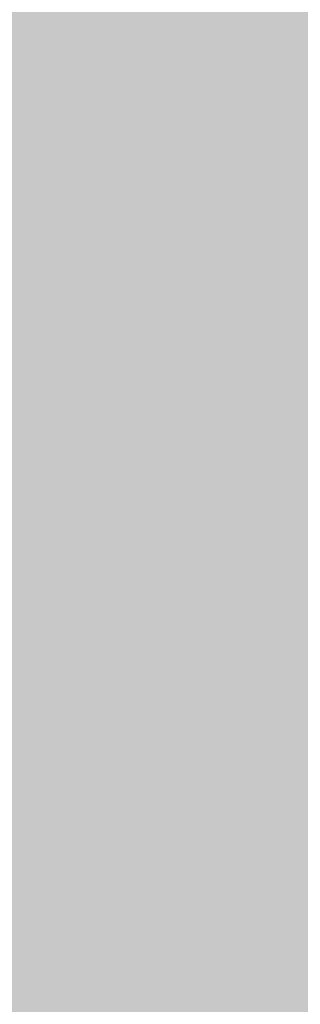
# Model space of a CAD drawing. Units: inches. Extents: x 2083 to 3317, y 1141 to 2115.
# Tile 187 of 256: x 3126.8176 to 3126.8914, y 1263.3548 to 1263.6134. Entities that reach past the tile are written whole.
import ezdxf

# ---------------------------------------------------------------- set-up
doc = ezdxf.new("R2010")
doc.units = ezdxf.units.IN
doc.layers.add('A-ANNO-DIMS', color=2, linetype='Continuous', lineweight=18)
doc.layers.add('A-WALL-PATT', color=251, linetype='Continuous', lineweight=13, true_color=0x636466)
doc.styles.get("Standard").update_dxf_attribs({"font": 'arial.ttf'})
doc.dimstyles.new('ISO-25', dxfattribs={"dimtxt": 12, "dimasz": 12, "dimexe": 1.25, "dimexo": 0.625, "dimtad": 1, "dimlunit": 3, "dimtxsty": 'Standard', "dimcen": 2.5, "dimadec": 0, "dimazin": 0, "dimtfac": 1, "dimtmove": 0, "dimatfit": 3, "dimfxl": 1, "dimarcsym": 0})

# ---------------------------------------------------------------- blocks, each defined once
blk = doc.blocks.new('*D26')
at = {"layer": 'A-ANNO-DIMS', "color": 0, "lineweight": -2, "transparency": 16777216}
for p, q in [((3088.98584, 1274.91509), (3088.98584, 1270.95196)), ((3111.24004, 1274.91509), (3111.24004, 1270.95196)), ((3076.98584, 1272.20196), (2840.26245, 1272.20196)), ((3111.24004, 1272.20196), (3088.98584, 1272.20196)), ((3123.24004, 1272.20196), (3135.24004, 1272.20196))]:
    blk.add_line(p, q, dxfattribs=at)
at = {"layer": 'A-ANNO-DIMS', "color": 0, "transparency": 16777216}
for points in [[(3076.98584, 1274.20196), (3076.98584, 1270.20196), (3088.98584, 1272.20196)], [(3123.24004, 1274.20196), (3123.24004, 1270.20196), (3111.24004, 1272.20196)]]:
    blk.add_solid(points, dxfattribs=at)
at = {"layer": 'Defpoints', "color": 0, "transparency": 16777216}
for p in [(3088.98584, 1275.54009), (3111.24004, 1275.54009), (3088.98584, 1272.20196)]:
    blk.add_point(p, dxfattribs=at)
at = {"layer": 'A-ANNO-DIMS', "color": 0, "transparency": 16777216, "insert": (2952.62415, 1279.0316), "char_height": 12, "attachment_point": 5}
blk.add_mtext('NIGHTSTAND 1\'-10 1/2" TYP.', dxfattribs=at)
blk = doc.blocks.new('*D27')
at = {"layer": 'A-ANNO-DIMS', "color": 0, "lineweight": -2, "transparency": 16777216}
for p, q in [((3114.57817, 1309.79428), (3114.57817, 1321.79428)), ((3111.86504, 1297.79428), (3115.82817, 1297.79428)), ((3114.57817, 1297.79428), (3114.57817, 1275.54009)), ((3111.86504, 1275.54009), (3115.82817, 1275.54009)), ((3114.57817, 1263.54009), (3114.57817, 1140.98859))]:
    blk.add_line(p, q, dxfattribs=at)
at = {"layer": 'A-ANNO-DIMS', "color": 0, "transparency": 16777216}
for points in [[(3112.57817, 1309.79428), (3116.57817, 1309.79428), (3114.57817, 1297.79428)], [(3112.57817, 1263.54009), (3116.57817, 1263.54009), (3114.57817, 1275.54009)]]:
    blk.add_solid(points, dxfattribs=at)
at = {"layer": 'Defpoints', "color": 0, "transparency": 16777216}
for p in [(3111.24004, 1297.79428), (3111.24004, 1275.54009), (3114.57817, 1275.54009)]:
    blk.add_point(p, dxfattribs=at)
at = {"layer": 'A-ANNO-DIMS', "color": 0, "transparency": 16777216, "insert": (3107.74853, 1196.26434), "char_height": 12, "attachment_point": 5, "rotation": 90}
blk.add_mtext('1\'-10 1/2" TYP.', dxfattribs=at)

msp = doc.modelspace()

# ---------------------------------------------------------------- hatches: boundary and pattern name
at = {"layer": 'A-WALL-PATT'}
h = msp.add_hatch(color=256, dxfattribs=at)
h.dxf.hatch_style = 1
h.paths.add_polyline_path([(3126.95978, 2020.76136), (2748.95978, 2020.76136), (2604.95978, 2020.76136), (2226.95978, 2020.76136), (2226.95978, 1702.76136), (2466.95978, 1702.76136), (2466.95978, 1582.76136), (2418.95978, 1582.76136), (2418.95978, 1477.76136), (2226.95978, 1477.76136), (2226.95978, 1263.26136), (2544.95978, 1263.26136), (2544.95978, 1411.76136), (2604.95978, 1411.76136), (2685.95978, 1411.76136), (2685.95978, 1420.76136), (2604.95978, 1420.76136), (2604.95978, 1573.76136), (2604.95978, 1702.76136), (2604.95978, 2011.76136), (2748.95978, 2011.76136), (2748.95978, 1702.76136), (2862.95978, 1702.76136), (2862.95978, 1621.76136), (2871.95978, 1621.76136), (2871.95978, 1702.76136), (2883.95978, 1702.76136), (2883.95978, 1706.93946, -0.026459), (2883.95978, 1711.76136), (2757.95978, 1711.76136), (2757.95978, 1807.76136), (2787.95978, 1807.76136), (2787.95978, 1812.26136), (2757.95978, 1812.26136), (2757.95978, 2011.76136), (2877.95978, 2011.76136), (2877.95978, 1812.26136), (2847.95978, 1812.26136), (2847.95978, 1807.76136), (2889.83574, 1807.76136), (2889.83574, 1812.26136), (2882.45978, 1812.26136), (2882.45978, 2011.76136), (3117.95978, 2011.76136), (3117.95978, 1812.26136), (2937.83574, 1812.26136), (2937.83574, 1807.76136), (2995.70978, 1807.76136), (2995.70978, 1796.11767), (3000.20978, 1796.11767), (3000.20978, 1807.76136), (3117.95978, 1807.76136), (3117.95978, 1711.76136), (3000.20978, 1711.76136), (3000.20978, 1760.11767), (2998.5727, 1760.11767, -0.020711), (2995.70978, 1760.11767), (2995.70978, 1711.76136), (2931.95978, 1711.76136), (2931.95978, 1702.76136), (3126.95978, 1702.76136)])
h.paths.add_polyline_path([(2471.45978, 2011.76136), (2471.45978, 1810.01136), (2462.71694, 1810.01136), (2462.71694, 1805.51136), (2505.95978, 1805.51136), (2505.95978, 1810.01136), (2475.95978, 1810.01136), (2475.95978, 2011.76136), (2595.95978, 2011.76136), (2595.95978, 1810.01136), (2565.95978, 1810.01136), (2565.95978, 1805.51136), (2595.95978, 1805.51136), (2595.95978, 1711.76136), (2235.95978, 1711.76136), (2235.95978, 1805.51136), (2353.70978, 1805.51136), (2353.70978, 1796.05416), (2358.20978, 1796.05416), (2358.20978, 1805.51136), (2414.71694, 1805.51136), (2414.71694, 1810.01136), (2235.95978, 1810.01136), (2235.95978, 2011.76136)], flags=16)
h.paths.add_polyline_path([(2270.20473, 1994.61001), (2270.20473, 1970.61001), (2246.20473, 1970.61001), (2246.20473, 1994.61001)], flags=0)
edge = h.paths.add_edge_path(flags=0)
edge.add_ellipse((2332.02739, 1899.79818), major_axis=(-3.04299, 3.04299), ratio=0.1682525, start_angle=-161.33217, end_angle=-156.30711, ccw=False)
edge.add_ellipse((2333.08204, 1898.74353), major_axis=(-1.05465, 1.05465), ratio=0.4535321, start_angle=-123.37102, end_angle=-94.15911)
edge = h.paths.add_edge_path(flags=0)
edge.add_ellipse((2332.02739, 1968.87629), major_axis=(3.04299, 3.04299), ratio=0.1682525, start_angle=18.66783, end_angle=23.69289)
edge.add_spline(control_points=[(2332.9256, 1970.6911), (2332.22677, 1970.3361), (2330.89371, 1969.65891), (2328.41308, 1970.93214), (2327.20393, 1967.74871), (2324.7096, 1969.95559), (2322.53282, 1967.01235), (2320.01285, 1971.29581), (2317.68031, 1968.15784), (2316.04053, 1967.10205), (2315.4269, 1966.8096)], knot_values=[0, 0, 0, 0, 2.267059, 4.324559, 6.685584, 8.878641, 11.121502, 14.300359, 17.755284, 19.732645, 19.732645, 19.732645, 19.732645], degree=3, periodic=0)
edge.add_ellipse((2332.02739, 1968.87629), major_axis=(3.04299, 3.04299), ratio=0.1682525, start_angle=18.66783, end_angle=23.69289, ccw=False)
edge.add_ellipse((2333.08204, 1969.93094), major_axis=(1.05465, 1.05465), ratio=0.4535321, start_angle=56.62898, end_angle=85.84089, ccw=False)
edge = h.paths.add_edge_path(flags=0)
edge.add_spline(control_points=[(2296.42829, 1967.98791), (2293.6278, 1965.33631), (2287.70362, 1959.72709), (2299.74386, 1949.9957), (2294.53259, 1935.66853), (2290.57323, 1920.60351), (2293.39412, 1909.97369), (2296.18541, 1904.96654)], knot_values=[0.099185, 0.099185, 0.099185, 0.099185, 0.345301, 0.619822, 0.982653, 1.386093, 1.810555, 1.810555, 1.810555, 1.810555], degree=3, periodic=0)
edge.add_spline(control_points=[(2296.18541, 1904.96654), (2297.38358, 1902.6193), (2298.00097, 1901.94931), (2298.55297, 1901.46815)], knot_values=[0.006246, 0.006246, 0.006246, 0.006246, 0.055476, 0.055476, 0.055476, 0.055476], degree=3, periodic=0)
edge.add_spline(control_points=[(2298.55297, 1901.46815), (2297.25861, 1900.92322), (2295.22529, 1900.23213), (2293.06023, 1900.61421), (2292.10142, 1900.78841), (2292.08958, 1900.79057)], knot_values=[0.312835, 0.312835, 0.312835, 0.312835, 0.40178, 0.474987, 0.475903, 0.475903, 0.475903, 0.475903], degree=3, periodic=0)
edge.add_arc((2292.79365, 1904.66411), 3.93701, 215.4209, 259.69818, ccw=False)
edge.add_spline(control_points=[(2289.58531, 1902.3823), (2289.47665, 1902.53509), (2289.36848, 1902.68804), (2289.26086, 1902.84117)], knot_values=[0.102872, 0.102872, 0.102872, 0.102872, 0.116896, 0.116896, 0.116896, 0.116896], degree=3, periodic=0)
edge.add_spline(control_points=[(2289.26086, 1902.84117), (2288.6866, 1902.55019), (2287.64005, 1902.0199), (2285.88134, 1901.87395), (2283.85297, 1901.50435), (2281.71999, 1899.71054), (2278.46699, 1899.49294), (2276.15714, 1901.8832), (2272.25895, 1899.80407), (2267.77761, 1901.84318), (2262.24388, 1900.18403), (2257.41493, 1901.78206), (2254.31837, 1900.72612), (2253.17828, 1900.33734)], knot_values=[0, 0, 0, 0, 1.907977, 3.477176, 5.261074, 7.972851, 11.680248, 13.717921, 16.939592, 22.789562, 27.502503, 33.595215, 37.145618, 37.145618, 37.145618, 37.145618], degree=3, periodic=0)
edge.add_line((2253.17828, 1900.33734), (2250.24424, 1902.84117))
edge.add_line((2250.24424, 1902.84117), (2250.24424, 1965.8333))
edge.add_line((2250.24424, 1965.8333), (2253.17828, 1968.33712))
edge.add_spline(control_points=[(2253.17828, 1968.33712), (2254.31837, 1967.94835), (2257.41493, 1966.89241), (2262.24388, 1968.49043), (2267.77761, 1966.83128), (2271.52673, 1968.53722), (2273.87591, 1967.82829), (2274.2067, 1967.72764)], knot_values=[0, 0, 0, 0, 0.09018, 0.244935, 0.364644, 0.513233, 0.537855, 0.537855, 0.537855, 0.537855], degree=3, periodic=0)
edge.add_arc((2274.35289, 1963.79335), 3.93701, 72.05113, 92.12795, ccw=False)
edge.add_arc((2281.29693, 1985.23), 18.5963, 252.051134, 288.565722)
edge.add_arc((2292.31672, 1956.02888), 12.64608, 71.026788, 113.778218, ccw=False)
edge = h.paths.add_edge_path(flags=0)
edge.add_spline(control_points=[(2274.89941, 1951.85619), (2275.06616, 1951.61659), (2275.23269, 1951.37659), (2275.39799, 1951.13585)], knot_values=[1.409916, 1.409916, 1.409916, 1.409916, 1.43159, 1.43159, 1.43159, 1.43159], degree=3, periodic=0)
edge.add_spline(control_points=[(2275.39799, 1951.13585), (2275.79211, 1950.56189), (2276.17923, 1949.98377), (2276.54555, 1949.3971)], knot_values=[1.358238, 1.358238, 1.358238, 1.358238, 1.409916, 1.409916, 1.409916, 1.409916], degree=3, periodic=0)
edge.add_line((2276.54555, 1949.3971), (2277.43729, 1947.86218))
edge.add_spline(control_points=[(2277.43729, 1947.86218), (2276.30383, 1945.67311), (2274.6397, 1942.42688), (2274.63161, 1938.0939), (2272.79912, 1930.85155), (2274.35643, 1943.89705), (2275.94768, 1947.92336), (2276.54555, 1949.3971)], knot_values=[0.005632, 0.005632, 0.005632, 0.005632, 0.186014, 0.266002, 0.357087, 0.59639, 0.739732, 0.739732, 0.739732, 0.739732], degree=3, periodic=0)
edge.add_spline(control_points=[(2276.54555, 1949.3971), (2276.17923, 1949.98377), (2275.79211, 1950.56189), (2275.39799, 1951.13585)], knot_values=[1.358238, 1.358238, 1.358238, 1.358238, 1.409916, 1.409916, 1.409916, 1.409916], degree=3, periodic=0)
edge.add_spline(control_points=[(2275.39799, 1951.13585), (2274.9425, 1950.08045), (2274.20776, 1948.02527), (2273.9346, 1944.85148), (2272.46853, 1937.62749), (2273.46622, 1945.69647), (2274.70062, 1951.05947), (2274.89941, 1951.85619)], knot_values=[0.104364, 0.104364, 0.104364, 0.104364, 0.189636, 0.269624, 0.36071, 0.600013, 0.644622, 0.644622, 0.644622, 0.644622], degree=3, periodic=0)
h.paths.add_polyline_path([(2269.16751, 1963.12757, -0.357527), (2268.17063, 1960.97637, -0.092561), (2268.17063, 1939.43632, -0.357527), (2269.16751, 1937.28512, -0.357527), (2267.01631, 1938.282, -0.164785), (2254.68558, 1938.282, -0.357527), (2252.53438, 1937.28512, -0.357527), (2253.53126, 1939.43632, -0.092561), (2253.53126, 1960.97637, -0.357527), (2252.53438, 1963.12757, -0.357527), (2254.68558, 1962.13069, -0.164785), (2267.01631, 1962.13069, -0.357527)], flags=0)
h.paths.add_polyline_path([(2248.87407, 1967.8018), (2248.87407, 1957.02771), (2249.45778, 1957.02771), (2249.45778, 1911.64676), (2248.87407, 1911.64676), (2248.87407, 1900.87267), (2246.51186, 1900.87267, 0.197327), (2244.14966, 1902.45687), (2244.14966, 1966.21759, 0.197327), (2246.51186, 1967.8018)], flags=0)
h.paths.add_polyline_path([(2269.16751, 1931.38934, -0.357527), (2268.17063, 1929.23814, -0.092561), (2268.17063, 1907.6981, -0.357527), (2269.16751, 1905.54689, -0.357527), (2267.01631, 1906.54377, -0.164785), (2254.68558, 1906.54377, -0.357527), (2252.53438, 1905.54689, -0.357527), (2253.53126, 1907.6981, -0.092561), (2253.53126, 1929.23814, -0.357527), (2252.53438, 1931.38934, -0.357527), (2254.68558, 1930.39246, -0.164785), (2267.01631, 1930.39246, -0.357527)], flags=0)
edge = h.paths.add_edge_path(flags=0)
edge.add_spline(control_points=[(2276.19686, 1906.7237), (2276.16814, 1909.02893), (2276.11405, 1913.37185), (2270.59842, 1924.92498), (2273.90517, 1919.01278), (2275.92171, 1916.26206), (2275.47457, 1912.40215), (2277.25787, 1910.38062), (2276.69604, 1908.22504), (2276.64622, 1906.81302), (2276.61782, 1906.00841)], knot_values=[0, 0, 0, 0, 8.61026, 16.221274, 18.843057, 23.804898, 27.440828, 29.356102, 31.203478, 33.650687, 33.650687, 33.650687, 33.650687], degree=3, periodic=0)
edge.add_spline(control_points=[(2276.61782, 1906.00841), (2276.62331, 1905.62414), (2276.49774, 1904.62866), (2275.44178, 1903.85473), (2274.93731, 1903.08045), (2274.85908, 1902.84117)], knot_values=[0.156488, 0.156488, 0.156488, 0.156488, 0.184398, 0.231376, 0.250598, 0.250598, 0.250598, 0.250598], degree=3, periodic=0)
edge.add_line((2274.85908, 1902.84117), (2276.50598, 1902.84117))
edge.add_spline(control_points=[(2276.50598, 1902.84117), (2276.78831, 1903.08494), (2277.66507, 1904.1252), (2278.24954, 1904.34074), (2277.65387, 1908.52739), (2278.15567, 1906.22781), (2278.10046, 1905.28595), (2278.84667, 1904.06901), (2277.85679, 1903.41495), (2277.87419, 1902.99105), (2277.90356, 1902.84117)], knot_values=[0.059574, 0.059574, 0.059574, 0.059574, 0.080753, 0.103741, 0.16972, 0.176036, 0.207137, 0.240474, 0.262341, 0.27366, 0.27366, 0.27366, 0.27366], degree=3, periodic=0)
edge.add_line((2277.90356, 1902.84117), (2280.02983, 1902.84117))
edge.add_spline(control_points=[(2280.02983, 1902.84117), (2279.88822, 1903.0884), (2279.49926, 1903.98155), (2280.15228, 1905.93935), (2278.10362, 1909.65776), (2279.76239, 1907.18529), (2280.3279, 1904.87486), (2280.48511, 1903.48959), (2281.46327, 1903.24943), (2281.75834, 1902.9365), (2281.83404, 1902.84117)], knot_values=[0.013856, 0.013856, 0.013856, 0.013856, 0.034874, 0.088867, 0.107879, 0.126738, 0.158714, 0.193757, 0.217487, 0.226722, 0.226722, 0.226722, 0.226722], degree=3, periodic=0)
edge.add_spline(control_points=[(2281.83404, 1902.84117), (2281.78753, 1902.8267), (2281.64702, 1902.78299), (2281.39553, 1902.85949), (2281.08808, 1902.98524), (2280.72068, 1903.0609), (2280.33345, 1903.02573), (2280.12477, 1902.89888), (2280.02983, 1902.84117)], knot_values=[0, 0, 0, 0, 0.14413, 0.435517, 0.749276, 1.153046, 1.548371, 1.878348, 1.878348, 1.878348, 1.878348], degree=3, periodic=0)
edge.add_line((2280.02983, 1902.84117), (2277.90356, 1902.84117))
edge.add_spline(control_points=[(2277.90356, 1902.84117), (2277.89286, 1902.79586), (2277.8654, 1902.67964), (2277.60748, 1902.68748), (2277.27405, 1902.8007), (2276.83792, 1902.61977), (2276.58381, 1902.78926), (2276.50598, 1902.84117)], knot_values=[0, 0, 0, 0, 0.127189, 0.326199, 0.628009, 1.24357, 1.515331, 1.515331, 1.515331, 1.515331], degree=3, periodic=0)
edge.add_line((2276.50598, 1902.84117), (2274.85908, 1902.84117))
edge.add_spline(control_points=[(2274.85908, 1902.84117), (2274.81444, 1902.89859), (2274.72513, 1903.01345), (2274.49348, 1903.11897), (2274.24429, 1902.96054), (2273.93712, 1903.18494), (2273.61404, 1902.98314), (2273.40832, 1902.88304), (2273.32225, 1902.84117)], knot_values=[0, 0, 0, 0, 0.21843, 0.436957, 0.687977, 0.990379, 1.398396, 1.69185, 1.69185, 1.69185, 1.69185], degree=3, periodic=0)
edge.add_spline(control_points=[(2273.32225, 1902.84117), (2273.61674, 1903.44569), (2274.274, 1904.53825), (2276.02724, 1904.5737), (2276.20696, 1906.58364), (2276.19686, 1906.7237)], knot_values=[0.012227, 0.012227, 0.012227, 0.012227, 0.059472, 0.106218, 0.134458, 0.134458, 0.134458, 0.134458], degree=3, periodic=0)
h.paths.add_polyline_path([(2270.77605, 1897.78983), (2270.77605, 1873.78983), (2246.77605, 1873.78983), (2246.77605, 1897.78983)], flags=0)
h.paths.add_polyline_path([(2353.70978, 1760.00506), (2353.70978, 1760.05416), (2358.20978, 1760.05416, -0.033729)], flags=0)
h.paths.add_polyline_path([(2321.81912, 1737.52919), (2341.99533, 1737.52919, -0.414214), (2343.20327, 1736.32124), (2343.20327, 1721.0206, -0.414214), (2341.99533, 1719.81265), (2321.81912, 1719.81265, -0.414214), (2320.61117, 1721.0206), (2320.61117, 1736.32124, -0.414214)], flags=0)
h.paths.add_polyline_path([(2324.23501, 1736.32124), (2339.57944, 1736.32124, -0.414214), (2341.99533, 1733.90535), (2341.99533, 1725.44973, -0.414214), (2339.57944, 1723.03384), (2333.68059, 1723.03384), (2333.84532, 1722.04547, -0.870646), (2335.4254, 1721.82589, -0.767327), (2333.92269, 1721.42324), (2331.29102, 1721.42324, -0.767327), (2329.78832, 1721.82589, -0.870646), (2331.3684, 1722.04547), (2331.53313, 1723.03384), (2324.23501, 1723.03384, -0.414214), (2321.81912, 1725.44973), (2321.81912, 1733.90535, -0.414214)], flags=0)
h.paths.add_polyline_path([(2570.48379, 1928.61544), (2589.68379, 1928.61544), (2590.16883, 1928.61544), (2590.16883, 1904.9934), (2570.48379, 1904.9934)], flags=0)
h.paths.add_polyline_path([(2574.44732, 1927.26382, -1), (2572.82884, 1927.26382, -1)], flags=0)
h.paths.add_polyline_path([(2573.08987, 1926.94088), (2573.92503, 1927.77604), (2574.14774, 1927.55333), (2573.31258, 1926.71817)], flags=0)
h.paths.add_polyline_path([(2578.77906, 1919.72962, -1), (2571.59166, 1919.72962, -1)], flags=0)
h.paths.add_polyline_path([(2578.38536, 1919.72962, -1), (2571.98536, 1919.72962, -1)], flags=0)
h.paths.add_polyline_path([(2331.59576, 1729.47622, -1), (2333.61795, 1729.47622, -1)], flags=0)
h.paths.add_polyline_path([(2578.03423, 1927.26382, -1), (2576.41574, 1927.26382, -1)], flags=0)
h.paths.add_polyline_path([(2576.68885, 1927.53109), (2576.91156, 1927.7538), (2577.74673, 1926.91863), (2577.52402, 1926.69592)], flags=0)
h.paths.add_polyline_path([(2578.13906, 1909.85954, -1), (2572.23166, 1909.85954, -1)], flags=0)
h.paths.add_polyline_path([(2577.74536, 1909.85954, -1), (2572.62536, 1909.85954, -1)], flags=0)
h.paths.add_polyline_path([(2583.79772, 1927.26382, -1), (2582.17923, 1927.26382, -1)], flags=0)
h.paths.add_polyline_path([(2582.71865, 1927.7538), (2583.55381, 1926.91863), (2583.3311, 1926.69592), (2582.49594, 1927.53109)], flags=0)
h.paths.add_polyline_path([(2582.49594, 1927.53109), (2582.71865, 1927.7538), (2583.55381, 1926.91863), (2583.3311, 1926.69592)], flags=0)
h.paths.add_polyline_path([(2587.73906, 1920.52962, -1), (2581.83166, 1920.52962, -1)], flags=0)
h.paths.add_polyline_path([(2587.34536, 1920.52962, -1), (2582.22536, 1920.52962, -1)], flags=0)
h.paths.add_polyline_path([(2587.38462, 1927.26382, -1), (2585.76613, 1927.26382, -1)], flags=0)
h.paths.add_polyline_path([(2586.08199, 1926.98025), (2586.91716, 1927.81541), (2587.13987, 1927.5927), (2586.3047, 1926.75754)], flags=0)
h.paths.add_polyline_path([(2588.37906, 1910.65954, -1), (2581.19166, 1910.65954, -1)], flags=0)
h.paths.add_polyline_path([(2587.98536, 1910.65954, -1), (2581.58536, 1910.65954, -1)], flags=0)
h.paths.add_polyline_path([(2417.16773, 1729.4779), (2437.34394, 1729.4779, -0.414214), (2438.55188, 1728.26995), (2438.55188, 1712.96931, -0.414214), (2437.34394, 1711.76136), (2417.16773, 1711.76136, -0.414214), (2415.95978, 1712.96931), (2415.95978, 1728.26995, -0.414214)], flags=0)
h.paths.add_polyline_path([(2419.58362, 1728.26995), (2434.92805, 1728.26995, -0.414214), (2437.34394, 1725.85406), (2437.34394, 1717.39844, -0.414214), (2434.92805, 1714.98255), (2429.0292, 1714.98255), (2429.19393, 1713.99418, -0.870646), (2430.77401, 1713.7746, -0.767327), (2429.2713, 1713.37195), (2426.63963, 1713.37195, -0.767327), (2425.13693, 1713.7746, -0.870646), (2426.71701, 1713.99418), (2426.88174, 1714.98255), (2419.58362, 1714.98255, -0.414214), (2417.16773, 1717.39844), (2417.16773, 1725.85406, -0.414214)], flags=0)
h.paths.add_polyline_path([(2419.58362, 1728.26995), (2434.92805, 1728.26995, -0.414214), (2437.34394, 1725.85406), (2437.34394, 1717.39844, -0.414214), (2434.92805, 1714.98255), (2429.0292, 1714.98255), (2428.35812, 1719.00903), (2427.55282, 1719.00903), (2426.88174, 1714.98255), (2419.58362, 1714.98255, -0.414214), (2417.16773, 1717.39844), (2417.16773, 1725.85406, -0.414214)], flags=0)
h.paths.add_polyline_path([(2426.94437, 1721.42492, -1), (2428.96656, 1721.42492, -1)], flags=0)
h.paths.add_polyline_path([(2475.95978, 1702.76136), (2595.95978, 1702.76136), (2595.95978, 1582.76136), (2475.95978, 1582.76136)], flags=16)
h.paths.add_polyline_path([(2427.95978, 1573.76136), (2595.95978, 1573.76136), (2595.95978, 1468.76136), (2595.95978, 1420.76136), (2384.45978, 1420.76136), (2384.45978, 1468.76136), (2427.95978, 1468.76136)], flags=16)
h.paths.add_polyline_path([(2379.95978, 1468.76136), (2379.95978, 1420.76136), (2235.95978, 1420.76136), (2235.95978, 1468.76136)], flags=16)
h.paths.add_polyline_path([(2317.816, 1466.69577), (2337.9922, 1466.69577, -0.414214), (2339.20015, 1465.48782), (2339.20015, 1450.18718, -0.414214), (2337.9922, 1448.97923), (2317.816, 1448.97923, -0.414214), (2316.60805, 1450.18718), (2316.60805, 1465.48782, -0.414214)], flags=0)
h.paths.add_polyline_path([(2320.23189, 1465.48782), (2335.57631, 1465.48782, -0.414214), (2337.9922, 1463.07193), (2337.9922, 1454.61631, -0.414214), (2335.57631, 1452.20042), (2329.67747, 1452.20042), (2329.84219, 1451.21205, -0.870646), (2331.42228, 1450.99247, -0.767327), (2329.91957, 1450.58983), (2327.2879, 1450.58983, -0.767327), (2325.7852, 1450.99247, -0.870646), (2327.36528, 1451.21205), (2327.53001, 1452.20042), (2320.23189, 1452.20042, -0.414214), (2317.816, 1454.61631), (2317.816, 1463.07193, -0.414214)], flags=0)
h.paths.add_polyline_path([(2320.23189, 1465.48782), (2335.57631, 1465.48782, -0.414214), (2337.9922, 1463.07193), (2337.9922, 1454.61631, -0.414214), (2335.57631, 1452.20042), (2329.67747, 1452.20042), (2329.00638, 1456.22691), (2328.20109, 1456.22691), (2327.53001, 1452.20042), (2320.23189, 1452.20042, -0.414214), (2317.816, 1454.61631), (2317.816, 1463.07193, -0.414214)], flags=0)
h.paths.add_polyline_path([(2327.59264, 1458.6428, -1), (2329.61483, 1458.6428, -1)], flags=0)
h.paths.add_polyline_path([(2244.41174, 1433.34045), (2241.92094, 1433.34045, -0.414214), (2240.01786, 1435.24354), (2240.01786, 1440.95281, -0.414211), (2241.92093, 1442.8559), (2244.41174, 1442.8559, -1.976472)], flags=0)
h.paths.add_polyline_path([(2245.35689, 1434.39754, -0.414214), (2245.35689, 1441.79881, -2.144098)], flags=0)
h.paths.add_polyline_path([(2535.95978, 1416.26136), (2535.95978, 1272.26136), (2235.95978, 1272.26136), (2235.95978, 1416.26136)], flags=16)
h.paths.add_polyline_path([(2260.11956, 1384.29284), (2260.11956, 1362.03865), (2237.86537, 1362.03865), (2237.86537, 1384.29284)], flags=0)
edge = h.paths.add_edge_path(flags=0)
edge.add_line((2318.25185, 1362.0933), (2318.1458, 1362.00097))
edge.add_ellipse((2317.44512, 1360.43104), major_axis=(2.82164, 2.82164), ratio=0.1682525, start_angle=18.66783, end_angle=20.94813, ccw=False)
edge.add_ellipse((2318.42305, 1361.40897), major_axis=(0.97793, 0.97793), ratio=0.4535321, start_angle=56.62898, end_angle=70.2262, ccw=False)
edge = h.paths.add_edge_path(flags=0)
edge.add_line((2319.10737, 1295.57108), (2319.01504, 1295.67713))
edge.add_ellipse((2317.44512, 1296.37781), major_axis=(-2.82164, 2.82164), ratio=0.1682525, start_angle=-161.33217, end_angle=-159.05187, ccw=False)
edge.add_ellipse((2318.42305, 1295.39988), major_axis=(-0.97793, 0.97793), ratio=0.4535321, start_angle=-123.37102, end_angle=-109.7738)
edge = h.paths.add_edge_path(flags=0)
edge.add_spline(control_points=[(2284.21035, 1301.17022), (2284.58069, 1300.44472), (2284.89119, 1299.89202), (2285.15955, 1299.46102)], knot_values=[0.039066, 0.039066, 0.039066, 0.039066, 0.055476, 0.055476, 0.055476, 0.055476], degree=3, periodic=0)
edge.add_line((2285.15955, 1299.46102), (2284.21035, 1301.17022))
edge = h.paths.add_edge_path(flags=0)
edge.add_line((2280.41246, 1297.29801), (2283.36999, 1297.03612))
edge.add_line((2283.36999, 1297.03612), (2286.40569, 1297.92631))
edge.add_spline(control_points=[(2286.40569, 1297.92631), (2285.30549, 1297.46312), (2284.34478, 1297.12915), (2283.36999, 1297.03612)], knot_values=[0.394369, 0.394369, 0.394369, 0.394369, 0.475903, 0.475903, 0.475903, 0.475903], degree=3, periodic=0)
edge.add_spline(control_points=[(2283.36999, 1297.03612), (2283.28139, 1297.02767), (2282.31629, 1296.95734), (2281.3125, 1297.13448), (2280.42344, 1297.29602), (2280.41246, 1297.29801)], knot_values=[0.312835, 0.312835, 0.312835, 0.312835, 0.320246, 0.393453, 0.394369, 0.394369, 0.394369, 0.394369], degree=3, periodic=0)
edge = h.paths.add_edge_path(flags=0)
edge.add_line((2284.43556, 1359.60729), (2280.44629, 1355.32805))
edge.add_line((2280.44629, 1355.32805), (2279.57999, 1351.01775))
edge.add_line((2279.57999, 1351.01775), (2282.41297, 1346.58043))
edge.add_spline(control_points=[(2282.41297, 1346.58043), (2283.15333, 1345.58924), (2284.2529, 1344.0289), (2284.80104, 1342.38717), (2284.93516, 1341.80554)], knot_values=[1.240098, 1.240098, 1.240098, 1.240098, 1.332892, 1.382712, 1.382712, 1.382712, 1.382712], degree=3, periodic=0)
edge.add_spline(control_points=[(2284.93516, 1341.80554), (2285.31911, 1340.1406), (2285.23303, 1338.4092), (2284.90994, 1336.65412)], knot_values=[1.097484, 1.097484, 1.097484, 1.097484, 1.240098, 1.240098, 1.240098, 1.240098], degree=3, periodic=0)
edge.add_spline(control_points=[(2284.90994, 1336.65412), (2284.58685, 1334.89904), (2284.02675, 1333.12027), (2283.46264, 1331.36058)], knot_values=[0.95487, 0.95487, 0.95487, 0.95487, 1.097484, 1.097484, 1.097484, 1.097484], degree=3, periodic=0)
edge.add_line((2283.46264, 1331.36058), (2281.89038, 1326.15336))
edge.add_line((2281.89038, 1326.15336), (2280.75626, 1321.05609))
edge.add_line((2280.75626, 1321.05609), (2280.2992, 1316.00198))
edge.add_line((2280.2992, 1316.00198), (2280.71593, 1310.95007))
edge.add_line((2280.71593, 1310.95007), (2282.02809, 1305.97214))
edge.add_line((2282.02809, 1305.97214), (2284.21035, 1301.17022))
edge.add_spline(control_points=[(2284.21035, 1301.17022), (2283.34073, 1302.73019), (2282.6119, 1304.33649), (2282.02809, 1305.97214)], knot_values=[0.099185, 0.099185, 0.099185, 0.099185, 0.241799, 0.241799, 0.241799, 0.241799], degree=3, periodic=0)
edge.add_spline(control_points=[(2282.02809, 1305.97214), (2281.44428, 1307.60778), (2281.00549, 1309.27276), (2280.71593, 1310.95007)], knot_values=[0.241799, 0.241799, 0.241799, 0.241799, 0.384413, 0.384413, 0.384413, 0.384413], degree=3, periodic=0)
edge.add_spline(control_points=[(2280.71593, 1310.95007), (2280.43324, 1312.58761), (2280.28939, 1314.27696), (2280.29889, 1315.96203), (2280.2992, 1316.00198)], knot_values=[0.384413, 0.384413, 0.384413, 0.384413, 0.523647, 0.527028, 0.527028, 0.527028, 0.527028], degree=3, periodic=0)
edge.add_spline(control_points=[(2280.2992, 1316.00198), (2280.31233, 1317.68696), (2280.47787, 1319.36793), (2280.75626, 1321.05609)], knot_values=[0.527028, 0.527028, 0.527028, 0.527028, 0.669642, 0.669642, 0.669642, 0.669642], degree=3, periodic=0)
edge.add_spline(control_points=[(2280.75626, 1321.05609), (2281.03465, 1322.74425), (2281.42588, 1324.43961), (2281.89038, 1326.15336)], knot_values=[0.669642, 0.669642, 0.669642, 0.669642, 0.812256, 0.812256, 0.812256, 0.812256], degree=3, periodic=0)
edge.add_spline(control_points=[(2281.89038, 1326.15336), (2282.26438, 1327.53325), (2282.78787, 1329.26181), (2283.35275, 1331.01778), (2283.46264, 1331.36058)], knot_values=[0.812256, 0.812256, 0.812256, 0.812256, 0.927087, 0.95487, 0.95487, 0.95487, 0.95487], degree=3, periodic=0)
edge.add_line((2283.46264, 1331.36058), (2284.90994, 1336.65412))
edge.add_line((2284.90994, 1336.65412), (2284.93516, 1341.80554))
edge.add_line((2284.93516, 1341.80554), (2282.41297, 1346.58043))
edge.add_spline(control_points=[(2282.41297, 1346.58043), (2281.27513, 1348.10379), (2280.07845, 1349.57032), (2279.57999, 1351.01775)], knot_values=[1.382712, 1.382712, 1.382712, 1.382712, 1.525326, 1.525326, 1.525326, 1.525326], degree=3, periodic=0)
edge.add_spline(control_points=[(2279.57999, 1351.01775), (2279.44328, 1351.41472), (2279.13631, 1352.85692), (2279.73519, 1354.29039), (2280.44629, 1355.32805)], knot_values=[1.525326, 1.525326, 1.525326, 1.525326, 1.564439, 1.667941, 1.667941, 1.667941, 1.667941], degree=3, periodic=0)
edge.add_spline(control_points=[(2280.44629, 1355.32805), (2281.42611, 1356.75784), (2282.93084, 1358.18256), (2284.43556, 1359.60729)], knot_values=[1.667941, 1.667941, 1.667941, 1.667941, 1.810555, 1.810555, 1.810555, 1.810555], degree=3, periodic=0)
edge.add_arc((2280.62307, 1348.51818), 11.72618, 71.026788, 113.778218)
edge.add_arc((2270.40489, 1375.59516), 17.24357, 252.051134, 288.565722, ccw=False)
edge.add_arc((2263.96597, 1355.71785), 3.65062, 72.05113, 92.12795)
edge.add_arc((2263.96597, 1355.71785), 3.65062, 92.12795, 177.98513)
edge.add_spline(control_points=[(2260.3176, 1355.8462), (2260.26042, 1354.22067), (2260.55128, 1350.18655), (2262.99934, 1346.76625), (2264.47274, 1344.64902)], knot_values=[1.43159, 1.43159, 1.43159, 1.43159, 1.564144, 1.770695, 1.770695, 1.770695, 1.770695], degree=3, periodic=0)
edge.add_line((2264.47274, 1344.64902), (2264.93559, 1343.98253))
edge.add_spline(control_points=[(2263.80104, 1340.24811), (2263.84324, 1340.51409), (2264.06724, 1341.75647), (2264.51269, 1343.00245), (2264.93505, 1343.98108)], knot_values=[0.53657, 0.53657, 0.53657, 0.53657, 0.559349, 0.644622, 0.644622, 0.644622, 0.644622], degree=3, periodic=0)
edge.add_spline(control_points=[(2264.93505, 1343.98108), (2265.11777, 1343.71497), (2265.29888, 1343.44791), (2265.47676, 1343.17936)], knot_values=[1.384077, 1.384077, 1.384077, 1.384077, 1.409916, 1.409916, 1.409916, 1.409916], degree=3, periodic=0)
edge.add_spline(control_points=[(2265.47676, 1343.17936), (2265.65464, 1342.91082), (2265.8293, 1342.64081), (2265.99913, 1342.36881)], knot_values=[1.358238, 1.358238, 1.358238, 1.358238, 1.384077, 1.384077, 1.384077, 1.384077], degree=3, periodic=0)
edge.add_line((2265.99913, 1342.36881), (2266.82601, 1340.94555))
edge.add_spline(control_points=[(2266.82601, 1340.94555), (2268.8944, 1337.08969), (2271.39817, 1325.843), (2270.51616, 1310.56856), (2275.91938, 1301.86061), (2277.78951, 1299.19945)], knot_values=[0.116896, 0.116896, 0.116896, 0.116896, 0.472987, 1.050969, 1.313793, 1.313793, 1.313793, 1.313793], degree=3, periodic=0)
edge.add_spline(control_points=[(2277.78951, 1299.19945), (2277.83941, 1299.12845), (2277.88943, 1299.0575), (2277.93957, 1298.98658)], knot_values=[0.109884, 0.109884, 0.109884, 0.109884, 0.116896, 0.116896, 0.116896, 0.116896], degree=3, periodic=0)
edge.add_line((2277.93957, 1298.98658), (2277.78885, 1299.19911))
edge.add_spline(control_points=[(2277.78885, 1299.19911), (2277.25658, 1298.92941), (2276.28635, 1298.4379), (2275.03935, 1298.33442), (2274.38333, 1298.2389), (2274.21525, 1298.20934)], knot_values=[33.12187, 33.12187, 33.12187, 33.12187, 35.029056, 36.598255, 37.144827, 37.144827, 37.144827, 37.144827], degree=3, periodic=0)
edge.add_line((2274.21525, 1298.20934), (2273.07315, 1297.89296))
edge.add_spline(control_points=[(2273.07315, 1297.89296), (2272.32294, 1297.57978), (2271.03915, 1296.51051), (2269.24839, 1296.22606), (2268.4231, 1296.37465)], knot_values=[26.532584, 26.532584, 26.532584, 26.532584, 29.198919, 31.839101, 31.839101, 31.839101, 31.839101], degree=3, periodic=0)
edge.add_line((2268.4231, 1296.37465), (2263.8785, 1297.45753))
edge.add_spline(control_points=[(2263.8785, 1297.45753), (2263.55608, 1297.35943), (2261.86031, 1296.83869), (2260.23878, 1297.28241), (2258.93345, 1297.51646)], knot_values=[15.919551, 15.919551, 15.919551, 15.919551, 16.939592, 21.226067, 21.226067, 21.226067, 21.226067], degree=3, periodic=0)
edge.add_line((2258.93345, 1297.51646), (2254.05523, 1297.32901))
edge.add_spline(control_points=[(2254.05523, 1297.32901), (2253.75553, 1297.29582), (2252.11368, 1297.16517), (2250.46187, 1297.54422), (2249.12969, 1297.66788)], knot_values=[5.306517, 5.306517, 5.306517, 5.306517, 6.276435, 10.613034, 10.613034, 10.613034, 10.613034], degree=3, periodic=0)
edge.add_line((2249.12969, 1297.66788), (2244.33165, 1296.87776))
edge.add_line((2244.33165, 1296.87776), (2241.61103, 1299.19945))
edge.add_line((2241.61103, 1299.19945), (2241.61103, 1357.6094))
edge.add_line((2241.61103, 1357.6094), (2244.33165, 1359.9311))
edge.add_line((2244.33165, 1359.9311), (2252.72882, 1359.54269))
edge.add_spline(control_points=[(2252.72882, 1359.54269), (2252.87094, 1359.54644), (2253.30574, 1359.54817), (2253.73984, 1359.51427), (2254.03174, 1359.48243)], knot_values=[0.233291, 0.233291, 0.233291, 0.233291, 0.244935, 0.268927, 0.268927, 0.268927, 0.268927], degree=3, periodic=0)
edge.add_line((2254.03174, 1359.48243), (2259.58719, 1359.41639))
edge.add_spline(control_points=[(2259.58719, 1359.41639), (2260.67707, 1359.6285), (2262.0732, 1359.897), (2263.52369, 1359.45928), (2263.83042, 1359.36595)], knot_values=[0.422516, 0.422516, 0.422516, 0.422516, 0.513233, 0.537855, 0.537855, 0.537855, 0.537855], degree=3, periodic=0)
edge.add_arc((2263.96597, 1355.71785), 3.65062, 72.05113, 92.12795, ccw=False)
edge.add_arc((2270.40489, 1375.59516), 17.24357, 252.051134, 288.565722)
edge.add_arc((2280.62307, 1348.51818), 11.72618, 71.026788, 113.778218, ccw=False)
h.paths.add_polyline_path([(2240.34053, 1359.43471), (2240.34053, 1349.44435), (2240.88178, 1349.44435), (2240.88178, 1307.3645), (2240.34053, 1307.3645), (2240.34053, 1297.37414), (2238.15016, 1297.37414, 0.197327), (2235.95978, 1298.84311), (2235.95978, 1357.96575, 0.197327), (2238.15016, 1359.43471)], flags=0)
h.paths.add_polyline_path([(2259.15779, 1355.1005, -0.357527), (2258.23342, 1353.10578, -0.092561), (2258.23342, 1333.1326, -0.357527), (2259.15779, 1331.13788, -0.357527), (2257.16307, 1332.06225, -0.164785), (2245.7293, 1332.06225, -0.357527), (2243.73458, 1331.13788, -0.357527), (2244.65895, 1333.1326, -0.092561), (2244.65895, 1353.10578, -0.357527), (2243.73458, 1355.1005, -0.357527), (2245.7293, 1354.17613, -0.164785), (2257.16307, 1354.17613, -0.357527)], flags=0)
edge = h.paths.add_edge_path(flags=0)
edge.add_line((2265.99913, 1342.36881), (2266.82601, 1340.94555))
edge.add_line((2266.82601, 1340.94555), (2265.30756, 1337.81407))
edge.add_line((2265.30756, 1337.81407), (2264.35823, 1334.65294))
edge.add_line((2264.35823, 1334.65294), (2264.26201, 1333.7997))
edge.add_spline(control_points=[(2264.26201, 1333.7997), (2264.20836, 1333.18705), (2264.16206, 1332.36553), (2264.00714, 1331.41393), (2263.96905, 1331.20183)], knot_values=[0.464444, 0.464444, 0.464444, 0.464444, 0.516691, 0.531608, 0.531608, 0.531608, 0.531608], degree=3, periodic=0)
edge.add_spline(control_points=[(2263.96905, 1331.20183), (2263.77453, 1330.11887), (2263.42437, 1328.79084), (2263.25742, 1328.53065), (2263.23403, 1328.51461)], knot_values=[0.372682, 0.372682, 0.372682, 0.372682, 0.44885, 0.464444, 0.464444, 0.464444, 0.464444], degree=3, periodic=0)
edge.add_spline(control_points=[(2263.23403, 1328.51461), (2263.09638, 1328.42023), (2263.13117, 1329.30148), (2263.27495, 1330.61575)], knot_values=[0.280919, 0.280919, 0.280919, 0.280919, 0.372682, 0.372682, 0.372682, 0.372682], degree=3, periodic=0)
edge.add_spline(control_points=[(2263.27495, 1330.61575), (2263.41874, 1331.93002), (2263.67152, 1333.67732), (2263.96985, 1335.31503)], knot_values=[0.189157, 0.189157, 0.189157, 0.189157, 0.280919, 0.280919, 0.280919, 0.280919], degree=3, periodic=0)
edge.add_spline(control_points=[(2263.96985, 1335.31503), (2264.1005, 1336.03219), (2264.41878, 1337.62191), (2264.75485, 1338.86443), (2264.94742, 1339.49112)], knot_values=[0.097394, 0.097394, 0.097394, 0.097394, 0.137578, 0.189157, 0.189157, 0.189157, 0.189157], degree=3, periodic=0)
edge.add_spline(control_points=[(2264.94742, 1339.49112), (2265.29002, 1340.60605), (2265.64424, 1341.494), (2265.99913, 1342.36881)], knot_values=[0.005632, 0.005632, 0.005632, 0.005632, 0.097394, 0.097394, 0.097394, 0.097394], degree=3, periodic=0)
h.paths.add_polyline_path([(2259.15779, 1325.67097, -0.357527), (2258.23342, 1323.67625, -0.092561), (2258.23342, 1303.70307, -0.357527), (2259.15779, 1301.70835, -0.357527), (2257.16307, 1302.63272, -0.164785), (2245.7293, 1302.63272, -0.357527), (2243.73458, 1301.70835, -0.357527), (2244.65895, 1303.70307, -0.092561), (2244.65895, 1323.67625, -0.357527), (2243.73458, 1325.67097, -0.357527), (2245.7293, 1324.74661, -0.164785), (2257.16307, 1324.74661, -0.357527)], flags=0)
edge = h.paths.add_edge_path(flags=0)
edge.add_spline(control_points=[(2261.70894, 1317.31142), (2261.67948, 1317.41758), (2261.76186, 1317.38853), (2262.49074, 1316.08987), (2262.96218, 1315.3009)], knot_values=[14.955861, 14.955861, 14.955861, 14.955861, 16.221274, 18.694826, 18.694826, 18.694826, 18.694826], degree=3, periodic=0)
edge.add_spline(control_points=[(2262.96218, 1315.3009), (2262.99044, 1315.25362), (2263.7021, 1314.06738), (2264.34898, 1313.12715), (2264.73005, 1312.16415)], knot_values=[18.694826, 18.694826, 18.694826, 18.694826, 18.843057, 22.433791, 22.433791, 22.433791, 22.433791], degree=3, periodic=0)
edge.add_spline(control_points=[(2264.73005, 1312.16415), (2264.87556, 1311.79644), (2265.17687, 1310.76981), (2265.14307, 1309.55926), (2265.24774, 1308.82419)], knot_values=[22.433791, 22.433791, 22.433791, 22.433791, 23.804898, 26.172756, 26.172756, 26.172756, 26.172756], degree=3, periodic=0)
edge.add_line((2265.24774, 1308.82419), (2265.85077, 1307.17189))
edge.add_spline(control_points=[(2265.85077, 1307.17189), (2266.06502, 1306.82168), (2266.38439, 1306.33225), (2266.4244, 1305.78055), (2266.42037, 1305.61122)], knot_values=[28.062562, 28.062562, 28.062562, 28.062562, 29.356102, 29.911721, 29.911721, 29.911721, 29.911721], degree=3, periodic=0)
edge.add_spline(control_points=[(2266.42037, 1305.61122), (2266.41612, 1305.43259), (2266.394, 1305.25), (2266.36478, 1305.06586)], knot_values=[29.911721, 29.911721, 29.911721, 29.911721, 30.497837, 30.497837, 30.497837, 30.497837], degree=3, periodic=0)
edge.add_line((2266.36478, 1305.06586), (2266.06615, 1302.1363))
edge.add_spline(control_points=[(2266.06615, 1302.1363), (2266.07124, 1301.77998), (2265.99808, 1301.19998), (2265.66327, 1300.75896), (2265.50891, 1300.58588)], knot_values=[0.156488, 0.156488, 0.156488, 0.156488, 0.184398, 0.203543, 0.203543, 0.203543, 0.203543], degree=3, periodic=0)
edge.add_line((2265.50891, 1300.58588), (2264.43534, 1299.19945))
edge.add_line((2264.43534, 1299.19945), (2265.96244, 1299.19945))
edge.add_line((2265.96244, 1299.19945), (2267.33599, 1301.17528))
edge.add_line((2267.33599, 1301.17528), (2267.31167, 1301.98624))
edge.add_spline(control_points=[(2267.31167, 1301.98624), (2267.26111, 1302.8624), (2267.16021, 1303.73713), (2267.27149, 1303.3259)], knot_values=[0.126229, 0.126229, 0.126229, 0.126229, 0.166617, 0.166617, 0.166617, 0.166617], degree=3, periodic=0)
edge.add_spline(control_points=[(2267.27149, 1303.3259), (2267.28003, 1303.2943), (2267.30979, 1303.17537), (2267.37345, 1302.88361), (2267.40612, 1302.68283), (2267.41793, 1302.60103)], knot_values=[0.166617, 0.166617, 0.166617, 0.166617, 0.16972, 0.176036, 0.180765, 0.180765, 0.180765, 0.180765], degree=3, periodic=0)
edge.add_spline(control_points=[(2267.74389, 1300.9875), (2267.68758, 1301.15094), (2267.48052, 1301.65666), (2267.48375, 1302.14479), (2267.41793, 1302.60103)], knot_values=[0.180765, 0.180765, 0.180765, 0.180765, 0.193767, 0.220139, 0.220139, 0.220139, 0.220139], degree=3, periodic=0)
edge.add_line((2267.41793, 1302.60103), (2267.74389, 1300.9875))
edge.add_spline(control_points=[(2267.74389, 1300.9875), (2267.83196, 1300.73188), (2267.93202, 1300.3099), (2267.55484, 1299.97452), (2267.42937, 1299.82921)], knot_values=[0.220139, 0.220139, 0.220139, 0.220139, 0.240474, 0.25489, 0.25489, 0.25489, 0.25489], degree=3, periodic=0)
edge.add_line((2267.42937, 1299.82921), (2267.25836, 1299.19945))
edge.add_line((2267.25836, 1299.19945), (2269.22996, 1299.19945))
edge.add_spline(control_points=[(2269.22996, 1299.19945), (2269.09865, 1299.42869), (2268.84277, 1300.01625), (2269.01157, 1300.91592), (2268.9468, 1301.66074)], knot_values=[0.013856, 0.013856, 0.013856, 0.013856, 0.034874, 0.067073, 0.067073, 0.067073, 0.067073], degree=3, periodic=0)
edge.add_line((2268.9468, 1301.66074), (2268.43158, 1303.60311))
edge.add_spline(control_points=[(2268.43158, 1303.60311), (2268.1756, 1304.19237), (2267.59621, 1305.2513), (2268.0407, 1304.62321), (2268.25139, 1304.28242)], knot_values=[0.090155, 0.090155, 0.090155, 0.090155, 0.107879, 0.120289, 0.120289, 0.120289, 0.120289], degree=3, periodic=0)
edge.add_spline(control_points=[(2268.25139, 1304.28242), (2268.36088, 1304.10533), (2269.05775, 1302.91798), (2269.38269, 1301.59042), (2269.52141, 1300.77593), (2269.57522, 1300.55578)], knot_values=[0.120289, 0.120289, 0.120289, 0.120289, 0.126738, 0.158714, 0.173506, 0.173506, 0.173506, 0.173506], degree=3, periodic=0)
edge.add_line((2269.57522, 1300.55578), (2270.6858, 1299.42126))
edge.add_spline(control_points=[(2270.6858, 1299.42126), (2270.76722, 1299.35725), (2270.83785, 1299.2814), (2270.90292, 1299.19945)], knot_values=[0.21816, 0.21816, 0.21816, 0.21816, 0.226722, 0.226722, 0.226722, 0.226722], degree=3, periodic=0)
edge.add_line((2270.9372, 1299.19291), (2270.90292, 1299.19945))
edge.add_spline(control_points=[(2270.90292, 1299.19945), (2270.85981, 1299.18603), (2270.72951, 1299.1455), (2270.49631, 1299.21644), (2270.27166, 1299.30832), (2270.12102, 1299.34796), (2270.06334, 1299.35956)], knot_values=[0.939174, 0.939174, 0.939174, 0.939174, 1.083304, 1.374691, 1.68845, 1.878348, 1.878348, 1.878348, 1.878348], degree=3, periodic=0)
edge.add_line((2270.06334, 1299.35956), (2269.22996, 1299.19945))
edge.add_line((2269.22996, 1299.19945), (2267.25836, 1299.19945))
edge.add_spline(control_points=[(2267.25836, 1299.19945), (2267.24843, 1299.15743), (2267.22297, 1299.04967), (2266.98382, 1299.05694), (2266.80921, 1299.11623), (2266.6769, 1299.10909), (2266.63653, 1299.10481)], knot_values=[0.757665, 0.757665, 0.757665, 0.757665, 0.884854, 1.083864, 1.385675, 1.515331, 1.515331, 1.515331, 1.515331], degree=3, periodic=0)
edge.add_spline(control_points=[(2266.63653, 1299.10481), (2266.48522, 1299.08879), (2266.23581, 1299.01712), (2266.03461, 1299.15132), (2265.96244, 1299.19945)], knot_values=[0, 0, 0, 0, 0.485905, 0.757665, 0.757665, 0.757665, 0.757665], degree=3, periodic=0)
edge.add_line((2265.96244, 1299.19945), (2264.43534, 1299.19945))
edge.add_line((2264.43534, 1299.19945), (2263.85844, 1299.36712))
edge.add_spline(control_points=[(2263.85844, 1299.36712), (2263.81894, 1299.37091), (2263.77953, 1299.38572), (2263.74013, 1299.4015)], knot_values=[0.845925, 0.845925, 0.845925, 0.845925, 0.978627, 0.978627, 0.978627, 0.978627], degree=3, periodic=0)
edge.add_line((2263.72179, 1299.39643), (2263.01031, 1299.19945))
edge.add_spline(control_points=[(2263.01031, 1299.19945), (2263.24579, 1299.68286), (2263.50603, 1300.12811), (2263.87349, 1300.40803)], knot_values=[0.012227, 0.012227, 0.012227, 0.012227, 0.052971, 0.052971, 0.052971, 0.052971], degree=3, periodic=0)
edge.add_spline(control_points=[(2263.87349, 1300.40803), (2263.93213, 1300.4527), (2264.08424, 1300.55298), (2264.25519, 1300.62422), (2264.35969, 1300.66475)], knot_values=[0.052971, 0.052971, 0.052971, 0.052971, 0.059472, 0.069086, 0.069086, 0.069086, 0.069086], degree=3, periodic=0)
edge.add_line((2264.35969, 1300.66475), (2265.1419, 1301.07777))
edge.add_line((2265.1419, 1301.07777), (2265.67581, 1302.79956))
edge.add_line((2265.67581, 1302.79956), (2265.5407, 1305.70407))
edge.add_line((2265.5407, 1305.70407), (2264.80307, 1309.32772))
edge.add_line((2264.80307, 1309.32772), (2263.04053, 1314.09179))
edge.add_spline(control_points=[(2263.04053, 1314.09179), (2262.38357, 1315.67144), (2261.79597, 1316.99775), (2261.70894, 1317.31142)], knot_values=[11.216896, 11.216896, 11.216896, 11.216896, 14.955861, 14.955861, 14.955861, 14.955861], degree=3, periodic=0)
h.paths.add_polyline_path([(2871.95978, 1416.26136), (2895.91005, 1416.26136), (2895.91005, 1420.76136), (2871.95978, 1420.76136), (2871.95978, 1501.76136), (2862.95978, 1501.76136), (2862.95978, 1420.76136), (2805.95978, 1420.76136), (2805.95978, 1411.76136), (2862.95978, 1411.76136), (2862.95978, 1263.26136), (3126.95978, 1263.26136), (3126.95978, 1411.76136), (3126.95978, 1486.76136), (2943.95978, 1486.76136), (2943.95978, 1477.76136), (2967.86031, 1477.76136), (2967.86031, 1420.76136), (2943.91005, 1420.76136), (2943.91005, 1416.26136), (3117.95978, 1416.26136), (3117.95978, 1420.76136), (2972.36031, 1420.76136), (2972.36031, 1477.76136), (3117.95978, 1477.76136), (3117.95978, 1420.76136), (3117.95978, 1272.26136), (2871.95978, 1272.26136)], flags=0)
h.paths.add_polyline_path([(2457.12563, 1485.94251), (2527.60265, 1485.94251), (2527.60265, 1537.6357), (2457.12563, 1537.6357)], flags=8)
h.paths.add_polyline_path([(2481.00506, 1609.9818), (2590.76582, 1609.9818), (2590.76582, 1682.00336), (2481.00506, 1682.00336)], flags=8)
h.paths.add_polyline_path([(2483.08502, 1729.12678), (2553.56205, 1729.12678), (2553.56205, 1780.81998), (2483.08502, 1780.81998)], flags=8)
h = msp.add_hatch(color=256, dxfattribs=at)
h.dxf.hatch_style = 1
h.paths.add_polyline_path([(3126.95978, 1486.76136), (2943.95978, 1486.76136), (2943.95978, 1477.76136), (2967.86031, 1477.76136), (2967.86031, 1420.76136), (2943.91005, 1420.76136), (2943.91005, 1416.26136), (3117.95978, 1416.26136), (3117.95978, 1420.76136), (2972.36031, 1420.76136), (2972.36031, 1477.76136), (3117.95978, 1477.76136), (3117.95978, 1420.76136), (3117.95978, 1272.26136), (2871.95978, 1272.26136), (2871.95978, 1416.26136), (2895.91005, 1416.26136), (2895.91005, 1420.76136), (2871.95978, 1420.76136), (2871.95978, 1501.76136), (2862.95978, 1501.76136), (2862.95978, 1420.76136), (2805.95978, 1420.76136), (2805.95978, 1411.76136), (2862.95978, 1411.76136), (2862.95978, 1263.26136), (3126.95978, 1263.26136), (3126.95978, 1411.76136)])

# ---------------------------------------------------------------- dimensions: what is measured, and where the dimension line sits
at = {"layer": 'A-ANNO-DIMS'}
for base, p1, p2, angle, text, picture, middle in [((3114.57817, 1275.54009), (3111.24004, 1297.79428), (3111.24004, 1275.54009), 270, '<> TYP.', '*D27', (3107.74853, 1196.26434)), ((3088.98584, 1272.20196), (3111.24004, 1275.54009), (3088.98584, 1275.54009), 180, 'NIGHTSTAND <> TYP.', '*D26', (2952.62415, 1279.0316))]:
    dim = msp.add_linear_dim(base=base, p1=p1, p2=p2, angle=angle, text=text, dimstyle='ISO-25', override={"dimdec": 1, "dimlfac": 1, "dimrnd": 0, "dimzin": 1, "dimdsep": 46, "dimlunit": 4, "dimfrac": 2}, dxfattribs=at)
    dim.commit()
    dim.dimension.update_dxf_attribs({"geometry": picture, "text_midpoint": middle})

doc.saveas('drawing.dxf')
